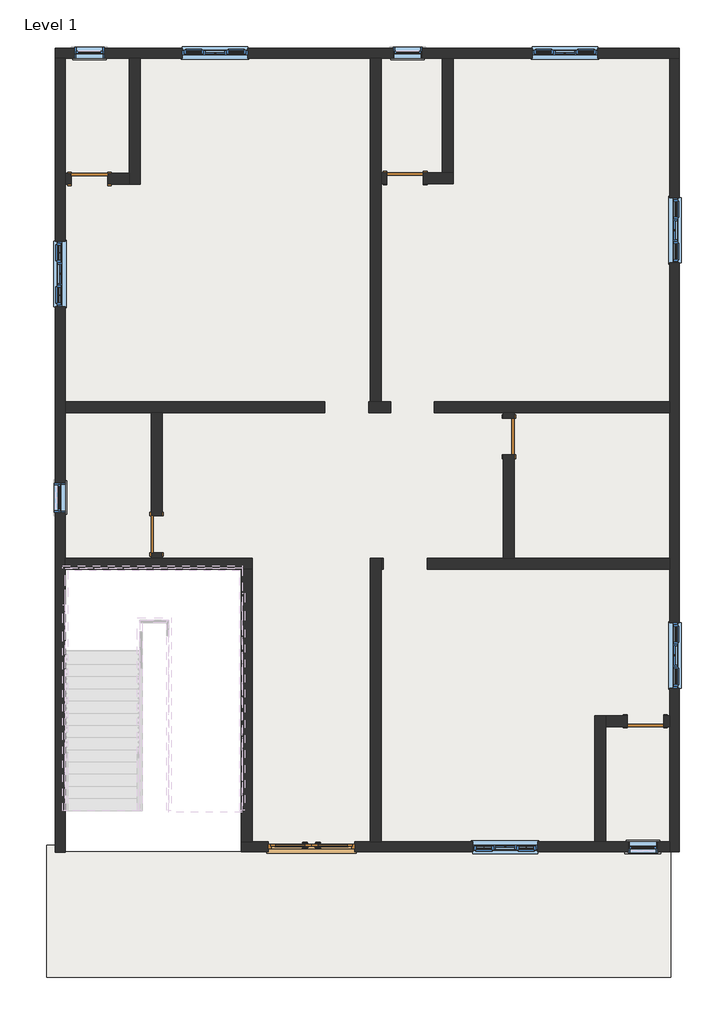
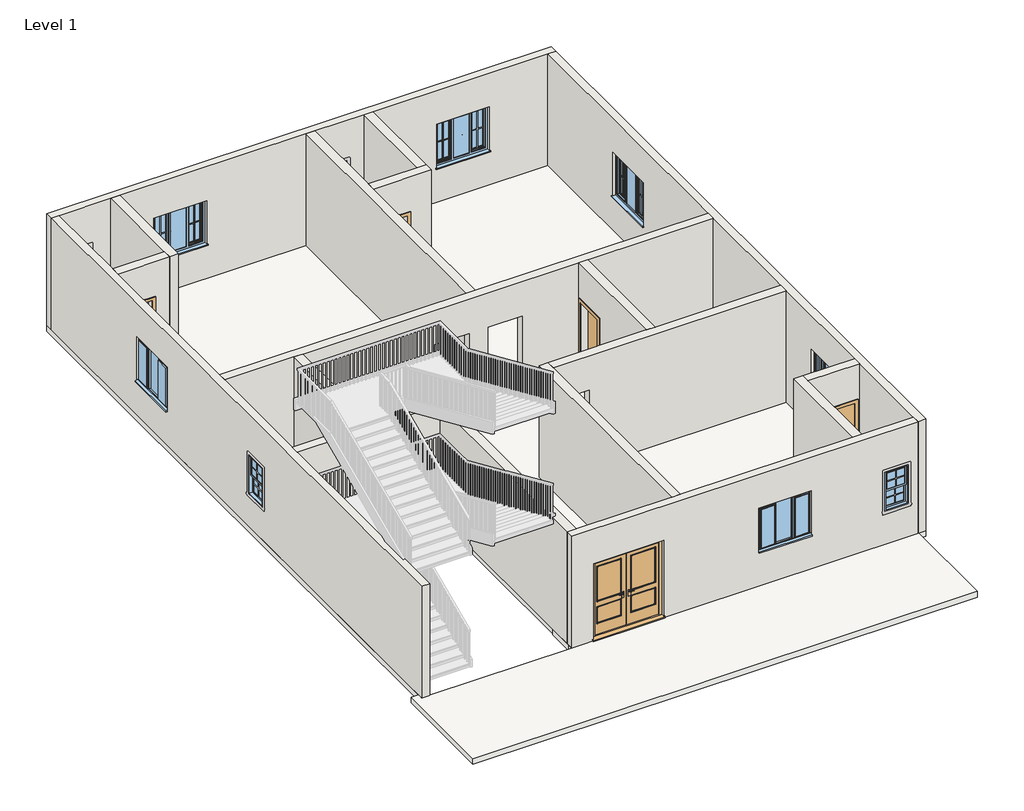
# One storey, part 1 of 6: 18 walls, 10 windows, 6 doors, 2 slabs.
"""IFC4 building model written with IfcOpenShell, lengths in millimetres."""

from ifc_helpers import new_model, si_unit, frame, origin, origin_with_axes, place, context, project, spatial, polyline, outline, extrude, faceted_brep, transform, mapped, element, save
from components import doors_extdbl_2_1810x2110mm_9ab1935a, doors_extdbl_2_1810x2110mm_b7024f51, door_85036156, window_679d2811, windows_tpl_w_glazing_cross_bars_1360x1210mm_0306471f

model = new_model("IFC4")

# Units and contexts
model_context = context("Model", 3, world=origin())
ifc_project = project(units=[si_unit("LENGTHUNIT", "METRE", prefix="MILLI")], contexts=[model_context])

# Site, building, storey
site = spatial("IfcSite", under=ifc_project)
building = spatial("IfcBuilding", under=site)
storey = spatial("IfcBuildingStorey", under=building, Name="Level 1", Elevation=0.0)

# Doors
placement = place(None, origin())
doors_extdbl_2_1810x2110mm_shape = doors_extdbl_2_1810x2110mm_9ab1935a(model_context)
doors_extdbl_2_1810x2110mm_2_shape = doors_extdbl_2_1810x2110mm_b7024f51(model_context)
element("IfcDoor", 1, ObjectType="Doors_ExtDbl_2 : 1810x2110mm", at=placement, inside=storey, context=model_context, shape_type="MappedRepresentation", body=[
    mapped(doors_extdbl_2_1810x2110mm_shape, transform((-2421.0852725, -7729.5064015, 0.0), x_axis=(1.0, 0.0, 0.0), y_axis=(0.0, 1.0, 0.0), z_axis=(0.0, 0.0, 1.0))),
    mapped(doors_extdbl_2_1810x2110mm_2_shape, transform((-2421.0852725, -7729.5064015, 0.0), x_axis=(1.0, 0.0, 0.0), y_axis=(0.0, 1.0, 0.0), z_axis=(0.0, 0.0, 1.0))),
])
door_shape = door_85036156(model_context)
element("IfcDoor", 2, ObjectType="Single-Flush : 30\" x 80\"", at=placement, inside=storey, context=model_context, shape_type="MappedRepresentation", body=[
    mapped(door_shape, transform((-7046.4415084, 6189.6935985, 0.0), x_axis=(-1.0, 0.0, 0.0), y_axis=(0.0, -1.0, 0.0), z_axis=(0.0, 0.0, 1.0))),
])
element("IfcDoor", 3, ObjectType="Single-Flush : 30\" x 80\"", at=placement, inside=storey, context=model_context, shape_type="MappedRepresentation", body=[
    mapped(door_shape, transform((-467.8415084, 6203.2000968, 0.0), x_axis=(-1.0, 0.0, 0.0), y_axis=(0.0, -1.0, 0.0), z_axis=(0.0, 0.0, 1.0))),
])
element("IfcDoor", 4, ObjectType="Single-Flush : 30\" x 80\"", at=placement, inside=storey, context=model_context, shape_type="MappedRepresentation", body=[
    mapped(door_shape, transform((-5649.4415084, -1217.2217109, 0.0), x_axis=(0.0, -1.0, 0.0), y_axis=(1.0, 0.0, 0.0), z_axis=(0.0, 0.0, 1.0))),
])
element("IfcDoor", 5, ObjectType="Single-Flush : 30\" x 80\"", at=placement, inside=storey, context=model_context, shape_type="MappedRepresentation", body=[
    mapped(door_shape, transform((1691.1584916, 817.5935985, 0.0), x_axis=(0.0, 1.0, 0.0), y_axis=(-1.0, 0.0, 0.0), z_axis=(0.0, 0.0, 1.0))),
])
element("IfcDoor", 6, ObjectType="Single-Flush : 30\" x 80\"", at=placement, inside=storey, context=model_context, shape_type="MappedRepresentation", body=[
    mapped(door_shape, transform((4535.9584916, -5113.3064015, 0.0), x_axis=(1.0, 0.0, 0.0), y_axis=(0.0, 1.0, 0.0), z_axis=(0.0, 0.0, 1.0))),
])

# Slabs
element("IfcSlab", 7, ObjectType="Generic - 12\"", at=placement, inside=storey, context=model_context, shape_type="SweptSolid", body=[
    extrude(outline(polyline([(5247.1584916, 8907.4935985), (5247.1584916, -7831.1064015), (-3879.0290366, -7831.1064015), (-3879.0290366, -6973.0610642), (-3866.3290366, -6973.0610642), (-3866.3290366, -1928.4217109), (-7554.4415084, -1928.4217109), (-7554.4415084, -7831.1064015), (-7757.6415084, -7831.1064015), (-7757.6415084, 8907.4935985), (5247.1584916, 8907.4935985)])), frame((0.0, 0.0, -152.4), z_axis=(0.0, 0.0, 1.0), x_axis=(1.0, 0.0, 0.0)), (0.0, 0.0, 1.0), 152.4),
])
element("IfcSlab", 8, ObjectType="Generic - 12\"", at=placement, inside=storey, context=model_context, shape_type="SweptSolid", body=[
    extrude(outline(polyline([(5063.8122085, -7701.6194881), (5063.8122085, -10451.1270757), (-7940.9877915, -10451.1270757), (-7940.9877915, -7701.6194881), (-7554.4415084, -7701.6194881), (-7554.4415084, -7831.1064015), (-3879.0290366, -7831.1064015), (-3879.0290366, -7701.6194881), (5063.8122085, -7701.6194881)])), frame((0.0, 0.0, -152.4), z_axis=(0.0, 0.0, 1.0), x_axis=(1.0, 0.0, 0.0)), (0.0, 0.0, 1.0), 152.4),
])

# Walls
element("IfcWall", 9, ObjectType="Generic - 4.5\"", at=placement, inside=storey, context=model_context, shape_type="Brep", body=[
    faceted_brep([(-1232.0415084, 1312.8935985, 2110.0), (-1232.0415084, 1312.8935985, 0.0), (-770.4415084, 1312.8935985, 0.0), (-770.4415084, 1312.8935985, 2110.0), (139.5584916, 1312.8935985, 2110.0), (139.5584916, 1312.8935985, 0.0), (1576.8584916, 1312.8935985, 0.0), (1805.4584916, 1312.8935985, 0.0), (5043.9584916, 1312.8935985, 0.0), (5043.9584916, 1312.8935985, 3048.0), (1805.4584916, 1312.8935985, 3048.0), (1576.8584916, 1312.8935985, 3048.0), (-5535.1415084, 1312.8935985, 3048.0), (-5763.7415084, 1312.8935985, 3048.0), (-7554.4415084, 1312.8935985, 3048.0), (-7554.4415084, 1312.8935985, 0.0), (-5763.7415084, 1312.8935985, 0.0), (-5535.1415084, 1312.8935985, 0.0), (-2142.0415084, 1312.8935985, 0.0), (-2142.0415084, 1312.8935985, 2110.0), (-770.4415084, 1541.4935985, 0.0), (-963.1415084, 1541.4935985, 0.0), (-1191.7415084, 1541.4935985, 0.0), (-1232.0415084, 1541.4935985, 0.0), (-1232.0415084, 1541.4935985, 2110.0), (-2142.0415084, 1541.4935985, 2110.0), (-2142.0415084, 1541.4935985, 0.0), (-7554.4415084, 1541.4935985, 0.0), (-7554.4415084, 1541.4935985, 3048.0), (-1191.7415084, 1541.4935985, 3048.0), (-963.1415084, 1541.4935985, 3048.0), (5043.9584916, 1541.4935985, 3048.0), (5043.9584916, 1541.4935985, 0.0), (139.5584916, 1541.4935985, 0.0), (139.5584916, 1541.4935985, 2110.0), (-770.4415084, 1541.4935985, 2110.0)], [[[0, 1, 2, 3, 4, 5, 6, 7, 8, 9, 10, 11, 12, 13, 14, 15, 16, 17, 18, 19]], [[20, 21, 22, 23, 24, 25, 26, 27, 28, 29, 30, 31, 32, 33, 34, 35]], [[33, 32, 8, 7, 6, 5]], [[2, 1, 23, 22, 21, 20]], [[18, 17, 16, 15, 27, 26]], [[14, 13, 12, 11, 10, 9, 31, 30, 29, 28]], [[9, 8, 32, 31]], [[15, 14, 28, 27]], [[5, 4, 34, 33]], [[3, 2, 20, 35]], [[4, 3, 35, 34]], [[26, 25, 19, 18]], [[24, 23, 1, 0]], [[25, 24, 0, 19]]]),
])
element("IfcWall", 10, ObjectType="Generic - 4.5\"", at=placement, inside=storey, context=model_context, shape_type="Brep", body=[
    faceted_brep([(-1191.7415084, 8704.2935985, 0.0), (-1191.7415084, 1541.4935985, 0.0), (-1191.7415084, 1541.4935985, 3048.0), (-1191.7415084, 8704.2935985, 3048.0), (-963.1415084, 8704.2935985, 0.0), (-963.1415084, 8704.2935985, 3048.0), (-963.1415084, 6317.5000968, 3048.0), (-963.1415084, 6088.9000968, 3048.0), (-963.1415084, 1541.4935985, 3048.0), (-963.1415084, 1541.4935985, 0.0), (-963.1415084, 6088.9000968, 0.0), (-963.1415084, 6317.5000968, 0.0)], [[[0, 1, 2, 3]], [[4, 5, 6, 7, 8, 9, 10, 11]], [[1, 0, 4, 11, 10, 9]], [[3, 2, 8, 7, 6, 5]], [[0, 3, 5, 4]], [[2, 1, 9, 8]]]),
])
element("IfcWall", 11, ObjectType="Generic - 4.5\"", at=placement, inside=storey, context=model_context, shape_type="Brep", body=[
    faceted_brep([(-6220.9415084, 8704.2935985, 0.0), (-6220.9415084, 6303.9935985, 0.0), (-6220.9415084, 6075.3935985, 0.0), (-6220.9415084, 6075.3935985, 3048.0), (-6220.9415084, 6303.9935985, 3048.0), (-6220.9415084, 8704.2935985, 3048.0), (-5992.3415084, 8704.2935985, 0.0), (-5992.3415084, 8704.2935985, 3048.0), (-5992.3415084, 6075.3935985, 3048.0), (-5992.3415084, 6075.3935985, 0.0)], [[[0, 1, 2, 3, 4, 5]], [[6, 7, 8, 9]], [[2, 1, 0, 6, 9]], [[5, 4, 3, 8, 7]], [[0, 5, 7, 6]], [[3, 2, 9, 8]]]),
])
element("IfcWall", 12, ObjectType="Generic - 4.5\"", at=placement, inside=storey, context=model_context, shape_type="SweptSolid", body=[
    extrude(outline(polyline([(0.0, -7554.4415084), (0.0, -7427.4415084), (2032.0, -7427.4415084), (2032.0, -6665.4415084), (0.0, -6665.4415084), (0.0, -6220.9415084), (3048.0, -6220.9415084), (3048.0, -7554.4415084), (0.0, -7554.4415084)])), frame((0.0, 6075.3935985, 0.0), z_axis=(0.0, 1.0, 0.0), x_axis=(0.0, 0.0, 1.0)), (0.0, 0.0, 1.0), 228.6),
])
element("IfcWall", 13, ObjectType="Generic - 4.5\"", at=placement, inside=storey, context=model_context, shape_type="Brep", body=[
    faceted_brep([(-963.1415084, 6088.9000968, 0.0), (-848.8415084, 6088.9000968, 0.0), (-848.8415084, 6088.9000968, 2032.0), (-86.8415084, 6088.9000968, 2032.0), (-86.8415084, 6088.9000968, 0.0), (535.4584916, 6088.9000968, 0.0), (535.4584916, 6088.9000968, 3048.0), (-963.1415084, 6088.9000968, 3048.0), (-848.8415084, 6317.5000968, 2032.0), (-848.8415084, 6317.5000968, 0.0), (-963.1415084, 6317.5000968, 0.0), (-963.1415084, 6317.5000968, 3048.0), (306.8584916, 6317.5000968, 3048.0), (535.4584916, 6317.5000968, 3048.0), (535.4584916, 6317.5000968, 0.0), (306.8584916, 6317.5000968, 0.0), (-86.8415084, 6317.5000968, 0.0), (-86.8415084, 6317.5000968, 2032.0)], [[[0, 1, 2, 3, 4, 5, 6, 7]], [[8, 9, 10, 11, 12, 13, 14, 15, 16, 17]], [[10, 9, 1, 0]], [[16, 15, 14, 5, 4]], [[7, 6, 13, 12, 11]], [[0, 7, 11, 10]], [[6, 5, 14, 13]], [[2, 1, 9, 8]], [[3, 2, 8, 17]], [[4, 3, 17, 16]]]),
])
element("IfcWall", 14, ObjectType="Generic - 4.5\"", at=placement, inside=storey, context=model_context, shape_type="SweptSolid", body=[
    extrude(outline(polyline([(535.4584916, 8704.2935985), (535.4584916, 6317.5000968), (306.8584916, 6317.5000968), (306.8584916, 8704.2935985), (535.4584916, 8704.2935985)])), origin_with_axes(), (0.0, 0.0, 1.0), 3048.0),
])
element("IfcWall", 15, ObjectType="Generic - 4.5\"", at=placement, inside=storey, context=model_context, shape_type="SweptSolid", body=[
    extrude(outline(polyline([(-1598.2217109, 2032.0), (-1598.2217109, 0.0), (-1712.5217109, 0.0), (-1712.5217109, 3048.0), (1312.8935985, 3048.0), (1312.8935985, 0.0), (-836.2217109, 0.0), (-836.2217109, 2032.0), (-1598.2217109, 2032.0)])), frame((-5763.7415084, 0.0, 0.0), z_axis=(1.0, 0.0, 0.0), x_axis=(0.0, 1.0, 0.0)), (0.0, 0.0, 1.0), 228.6),
])
element("IfcWall", 16, ObjectType="Generic - 4.5\"", at=placement, inside=storey, context=model_context, shape_type="Brep", body=[
    faceted_brep([(-7554.4415084, -1941.1217109, 0.0), (-3879.0290366, -1941.1217109, 0.0), (-3650.4290366, -1941.1217109, 0.0), (-3650.4290366, -1941.1217109, 3048.0), (-3879.0290366, -1941.1217109, 3048.0), (-7554.4415084, -1941.1217109, 3048.0), (-7554.4415084, -1712.5217109, 0.0), (-7554.4415084, -1712.5217109, 3048.0), (-5763.7415084, -1712.5217109, 3048.0), (-5535.1415084, -1712.5217109, 3048.0), (-3650.4290366, -1712.5217109, 3048.0), (-3650.4290366, -1712.5217109, 0.0), (-5535.1415084, -1712.5217109, 0.0), (-5763.7415084, -1712.5217109, 0.0)], [[[0, 1, 2, 3, 4, 5]], [[6, 7, 8, 9, 10, 11, 12, 13]], [[2, 1, 0, 6, 13, 12, 11]], [[5, 4, 3, 10, 9, 8, 7]], [[0, 5, 7, 6]], [[3, 2, 11, 10]]]),
])
element("IfcWall", 17, ObjectType="Generic - 4.5\"", at=placement, inside=storey, context=model_context, shape_type="SweptSolid", body=[
    extrude(outline(polyline([(-3879.0290366, -7627.9064015), (-3879.0290366, -1941.1217109), (-3650.4290366, -1941.1217109), (-3650.4290366, -7627.9064015), (-3879.0290366, -7627.9064015)])), origin_with_axes(), (0.0, 0.0, 1.0), 3048.0),
])
element("IfcWall", 18, ObjectType="Generic - 4.5\"", at=placement, inside=storey, context=model_context, shape_type="SweptSolid", body=[
    extrude(outline(polyline([(1312.8935985, 0.0), (1198.5935985, 0.0), (1198.5935985, 2032.0), (436.5935985, 2032.0), (436.5935985, 0.0), (-1712.5217109, 0.0), (-1712.5217109, 3048.0), (1312.8935985, 3048.0), (1312.8935985, 0.0)])), frame((1576.8584916, 0.0, 0.0), z_axis=(1.0, 0.0, 0.0), x_axis=(0.0, 1.0, 0.0)), (0.0, 0.0, 1.0), 228.6),
])
element("IfcWall", 19, ObjectType="Generic - 4.5\"", at=placement, inside=storey, context=model_context, shape_type="Brep", body=[
    faceted_brep([(-963.1415084, -7627.9064015, 0.0), (-963.1415084, -1941.1217109, 0.0), (-963.1415084, -1712.5217109, 0.0), (-963.1415084, -1712.5217109, 3048.0), (-963.1415084, -1941.1217109, 3048.0), (-963.1415084, -7627.9064015, 3048.0), (-1191.7415084, -7627.9064015, 0.0), (-1191.7415084, -7627.9064015, 3048.0), (-1191.7415084, -1712.5217109, 3048.0), (-1191.7415084, -1712.5217109, 0.0)], [[[0, 1, 2, 3, 4, 5]], [[6, 7, 8, 9]], [[2, 1, 0, 6, 9]], [[5, 4, 3, 8, 7]], [[0, 5, 7, 6]], [[3, 2, 9, 8]]]),
])
element("IfcWall", 20, ObjectType="Generic - 4.5\"", at=placement, inside=storey, context=model_context, shape_type="Brep", body=[
    faceted_brep([(-922.8415084, -1712.5217109, 2110.0), (-922.8415084, -1712.5217109, 0.0), (-963.1415084, -1712.5217109, 0.0), (-963.1415084, -1712.5217109, 3048.0), (1576.8584916, -1712.5217109, 3048.0), (1805.4584916, -1712.5217109, 3048.0), (5043.9584916, -1712.5217109, 3048.0), (5043.9584916, -1712.5217109, 0.0), (1805.4584916, -1712.5217109, 0.0), (1576.8584916, -1712.5217109, 0.0), (-12.8415084, -1712.5217109, 0.0), (-12.8415084, -1712.5217109, 2110.0), (-963.1415084, -1941.1217109, 0.0), (-922.8415084, -1941.1217109, 0.0), (-922.8415084, -1941.1217109, 2110.0), (-12.8415084, -1941.1217109, 2110.0), (-12.8415084, -1941.1217109, 0.0), (5043.9584916, -1941.1217109, 0.0), (5043.9584916, -1941.1217109, 3048.0), (-963.1415084, -1941.1217109, 3048.0)], [[[0, 1, 2, 3, 4, 5, 6, 7, 8, 9, 10, 11]], [[12, 13, 14, 15, 16, 17, 18, 19]], [[2, 1, 13, 12]], [[10, 9, 8, 7, 17, 16]], [[6, 5, 4, 3, 19, 18]], [[3, 2, 12, 19]], [[7, 6, 18, 17]], [[16, 15, 11, 10]], [[14, 13, 1, 0]], [[15, 14, 0, 11]]]),
])
element("IfcWall", 21, ObjectType="Generic - 4.5\"", at=placement, inside=storey, context=model_context, shape_type="Brep", body=[
    faceted_brep([(3710.4584916, -7627.9064015, 0.0), (3710.4584916, -5227.6064015, 0.0), (3710.4584916, -4999.0064015, 0.0), (3710.4584916, -4999.0064015, 3048.0), (3710.4584916, -5227.6064015, 3048.0), (3710.4584916, -7627.9064015, 3048.0), (3481.8584916, -7627.9064015, 0.0), (3481.8584916, -7627.9064015, 3048.0), (3481.8584916, -4999.0064015, 3048.0), (3481.8584916, -4999.0064015, 0.0)], [[[0, 1, 2, 3, 4, 5]], [[6, 7, 8, 9]], [[2, 1, 0, 6, 9]], [[5, 4, 3, 8, 7]], [[0, 5, 7, 6]], [[3, 2, 9, 8]]]),
])
element("IfcWall", 22, ObjectType="Generic - 4.5\"", at=placement, inside=storey, context=model_context, shape_type="SweptSolid", body=[
    extrude(outline(polyline([(2032.0, 4916.9584916), (0.0, 4916.9584916), (0.0, 5043.9584916), (3048.0, 5043.9584916), (3048.0, 3710.4584916), (0.0, 3710.4584916), (0.0, 4154.9584916), (2032.0, 4154.9584916), (2032.0, 4916.9584916)])), frame((0.0, -5227.6064015, 0.0), z_axis=(0.0, 1.0, 0.0), x_axis=(0.0, 0.0, 1.0)), (0.0, 0.0, 1.0), 228.6),
])
element("IfcWall", 23, ObjectType="Generic - 9\"", at=placement, inside=storey, context=model_context, shape_type="Brep", body=[
    faceted_brep([(-7757.6415084, 8704.2935985, 0.0), (-7554.4415084, 8704.2935985, 0.0), (-6220.9415084, 8704.2935985, 0.0), (-5992.3415084, 8704.2935985, 0.0), (-1191.7415084, 8704.2935985, 0.0), (-963.1415084, 8704.2935985, 0.0), (306.8584916, 8704.2935985, 0.0), (535.4584916, 8704.2935985, 0.0), (5043.9584916, 8704.2935985, 0.0), (5247.1584916, 8704.2935985, 0.0), (5247.1584916, 8704.2935985, 3048.0), (5043.9584916, 8704.2935985, 3048.0), (535.4584916, 8704.2935985, 3048.0), (306.8584916, 8704.2935985, 3048.0), (-963.1415084, 8704.2935985, 3048.0), (-1191.7415084, 8704.2935985, 3048.0), (-5992.3415084, 8704.2935985, 3048.0), (-6220.9415084, 8704.2935985, 3048.0), (-7554.4415084, 8704.2935985, 3048.0), (-7757.6415084, 8704.2935985, 3048.0), (2179.5584916, 8704.2935985, 2124.4), (3539.5584916, 8704.2935985, 2124.4), (3539.5584916, 8704.2935985, 914.4), (2179.5584916, 8704.2935985, 914.4), (-5110.2415084, 8704.2935985, 2124.4), (-3750.2415084, 8704.2935985, 2124.4), (-3750.2415084, 8704.2935985, 914.4), (-5110.2415084, 8704.2935985, 914.4), (-7351.2415084, 8704.2935985, 1981.2), (-6741.6415084, 8704.2935985, 1981.2), (-6741.6415084, 8704.2935985, 914.4), (-7351.2415084, 8704.2935985, 914.4), (-721.8415084, 8704.2935985, 1981.2), (-112.2415084, 8704.2935985, 1981.2), (-112.2415084, 8704.2935985, 914.4), (-721.8415084, 8704.2935985, 914.4), (-7757.6415084, 8907.4935985, 0.0), (-7757.6415084, 8907.4935985, 3048.0), (5247.1584916, 8907.4935985, 3048.0), (5247.1584916, 8907.4935985, 0.0), (2179.5584916, 8907.4935985, 2124.4), (2179.5584916, 8907.4935985, 914.4), (3539.5584916, 8907.4935985, 914.4), (3539.5584916, 8907.4935985, 2124.4), (-5110.2415084, 8907.4935985, 2124.4), (-5110.2415084, 8907.4935985, 914.4), (-3750.2415084, 8907.4935985, 914.4), (-3750.2415084, 8907.4935985, 2124.4), (-7351.2415084, 8907.4935985, 1981.2), (-7351.2415084, 8907.4935985, 914.4), (-6741.6415084, 8907.4935985, 914.4), (-6741.6415084, 8907.4935985, 1981.2), (-721.8415084, 8907.4935985, 1981.2), (-721.8415084, 8907.4935985, 914.4), (-112.2415084, 8907.4935985, 914.4), (-112.2415084, 8907.4935985, 1981.2)], [[[0, 1, 2, 3, 4, 5, 6, 7, 8, 9, 10, 11, 12, 13, 14, 15, 16, 17, 18, 19], [20, 21, 22, 23], [24, 25, 26, 27], [28, 29, 30, 31], [32, 33, 34, 35]], [[36, 37, 38, 39], [40, 41, 42, 43], [44, 45, 46, 47], [48, 49, 50, 51], [52, 53, 54, 55]], [[9, 8, 7, 6, 5, 4, 3, 2, 1, 0, 36, 39]], [[19, 18, 17, 16, 15, 14, 13, 12, 11, 10, 38, 37]], [[0, 19, 37, 36]], [[10, 9, 39, 38]], [[41, 40, 20, 23]], [[42, 41, 23, 22]], [[43, 42, 22, 21]], [[40, 43, 21, 20]], [[45, 44, 24, 27]], [[46, 45, 27, 26]], [[47, 46, 26, 25]], [[44, 47, 25, 24]], [[49, 48, 28, 31]], [[50, 49, 31, 30]], [[51, 50, 30, 29]], [[48, 51, 29, 28]], [[53, 52, 32, 35]], [[54, 53, 35, 34]], [[55, 54, 34, 33]], [[52, 55, 33, 32]]]),
])
element("IfcWall", 24, ObjectType="Generic - 9\"", at=placement, inside=storey, context=model_context, shape_type="Brep", body=[
    faceted_brep([(5043.9584916, 8704.2935985, 0.0), (5043.9584916, 1541.4935985, 0.0), (5043.9584916, 1312.8935985, 0.0), (5043.9584916, -1712.5217109, 0.0), (5043.9584916, -1941.1217109, 0.0), (5043.9584916, -4999.0064015, 0.0), (5043.9584916, -5227.6064015, 0.0), (5043.9584916, -7627.9064015, 0.0), (5043.9584916, -7831.1064015, 0.0), (5043.9584916, -7831.1064015, 3048.0), (5043.9584916, -7627.9064015, 3048.0), (5043.9584916, -5227.6064015, 3048.0), (5043.9584916, -4999.0064015, 3048.0), (5043.9584916, -1941.1217109, 3048.0), (5043.9584916, -1712.5217109, 3048.0), (5043.9584916, 1312.8935985, 3048.0), (5043.9584916, 1541.4935985, 3048.0), (5043.9584916, 8704.2935985, 3048.0), (5043.9584916, 5796.5435985, 2124.4), (5043.9584916, 4436.5435985, 2124.4), (5043.9584916, 4436.5435985, 914.4), (5043.9584916, 5796.5435985, 914.4), (5043.9584916, -3061.7064015, 2124.4), (5043.9584916, -4421.7064015, 2124.4), (5043.9584916, -4421.7064015, 914.4), (5043.9584916, -3061.7064015, 914.4), (5247.1584916, 8704.2935985, 0.0), (5247.1584916, 8704.2935985, 3048.0), (5247.1584916, -7831.1064015, 3048.0), (5247.1584916, -7831.1064015, 0.0), (5247.1584916, 5796.5435985, 2124.4), (5247.1584916, 5796.5435985, 914.4), (5247.1584916, 4436.5435985, 914.4), (5247.1584916, 4436.5435985, 2124.4), (5247.1584916, -3061.7064015, 2124.4), (5247.1584916, -3061.7064015, 914.4), (5247.1584916, -4421.7064015, 914.4), (5247.1584916, -4421.7064015, 2124.4)], [[[0, 1, 2, 3, 4, 5, 6, 7, 8, 9, 10, 11, 12, 13, 14, 15, 16, 17], [18, 19, 20, 21], [22, 23, 24, 25]], [[26, 27, 28, 29], [30, 31, 32, 33], [34, 35, 36, 37]], [[8, 7, 6, 5, 4, 3, 2, 1, 0, 26, 29]], [[9, 8, 29, 28]], [[17, 16, 15, 14, 13, 12, 11, 10, 9, 28, 27]], [[31, 30, 18, 21]], [[32, 31, 21, 20]], [[33, 32, 20, 19]], [[30, 33, 19, 18]], [[35, 34, 22, 25]], [[36, 35, 25, 24]], [[37, 36, 24, 23]], [[34, 37, 23, 22]], [[0, 17, 27, 26]]]),
])
element("IfcWall", 25, ObjectType="Generic - 9\"", at=placement, inside=storey, context=model_context, shape_type="Brep", body=[
    faceted_brep([(5043.9584916, -7627.9064015, 0.0), (3710.4584916, -7627.9064015, 0.0), (3481.8584916, -7627.9064015, 0.0), (-963.1415084, -7627.9064015, 0.0), (-1191.7415084, -7627.9064015, 0.0), (-1516.0852725, -7627.9064015, 0.0), (-1516.0852725, -7627.9064015, 2110.0), (-3326.0852725, -7627.9064015, 2110.0), (-3326.0852725, -7627.9064015, 0.0), (-3650.4290366, -7627.9064015, 0.0), (-3879.0290366, -7627.9064015, 0.0), (-3879.0290366, -7627.9064015, 3048.0), (-3650.4290366, -7627.9064015, 3048.0), (-1191.7415084, -7627.9064015, 3048.0), (-963.1415084, -7627.9064015, 3048.0), (3481.8584916, -7627.9064015, 3048.0), (3710.4584916, -7627.9064015, 3048.0), (5043.9584916, -7627.9064015, 3048.0), (2294.9584916, -7627.9064015, 2124.4), (934.9584916, -7627.9064015, 2124.4), (934.9584916, -7627.9064015, 914.4), (2294.9584916, -7627.9064015, 914.4), (4789.9584916, -7627.9064015, 1981.2), (4180.3584916, -7627.9064015, 1981.2), (4180.3584916, -7627.9064015, 914.4), (4789.9584916, -7627.9064015, 914.4), (-1516.0852725, -7831.1064015, 2110.0), (-1516.0852725, -7831.1064015, 0.0), (5043.9584916, -7831.1064015, 0.0), (5043.9584916, -7831.1064015, 3048.0), (-3879.0290366, -7831.1064015, 3048.0), (-3879.0290366, -7831.1064015, 0.0), (-3326.0852725, -7831.1064015, 0.0), (-3326.0852725, -7831.1064015, 2110.0), (2294.9584916, -7831.1064015, 2124.4), (2294.9584916, -7831.1064015, 914.4), (934.9584916, -7831.1064015, 914.4), (934.9584916, -7831.1064015, 2124.4), (4789.9584916, -7831.1064015, 1981.2), (4789.9584916, -7831.1064015, 914.4), (4180.3584916, -7831.1064015, 914.4), (4180.3584916, -7831.1064015, 1981.2)], [[[0, 1, 2, 3, 4, 5, 6, 7, 8, 9, 10, 11, 12, 13, 14, 15, 16, 17], [18, 19, 20, 21], [22, 23, 24, 25]], [[26, 27, 28, 29, 30, 31, 32, 33], [34, 35, 36, 37], [38, 39, 40, 41]], [[32, 31, 10, 9, 8]], [[28, 27, 5, 4, 3, 2, 1, 0]], [[17, 16, 15, 14, 13, 12, 11, 30, 29]], [[0, 17, 29, 28]], [[11, 10, 31, 30]], [[35, 34, 18, 21]], [[36, 35, 21, 20]], [[37, 36, 20, 19]], [[34, 37, 19, 18]], [[39, 38, 22, 25]], [[40, 39, 25, 24]], [[41, 40, 24, 23]], [[38, 41, 23, 22]], [[8, 7, 33, 32]], [[6, 5, 27, 26]], [[7, 6, 26, 33]]]),
])
element("IfcWall", 26, ObjectType="Generic - 9\"", at=placement, inside=storey, context=model_context, shape_type="Brep", body=[
    faceted_brep([(-7757.6415084, 8704.2935985, 0.0), (-7757.6415084, -7843.8064015, 0.0), (-7757.6415084, -7843.8064015, 3048.0), (-7757.6415084, 8704.2935985, 3048.0), (-7757.6415084, 3528.4935985, 2124.4), (-7757.6415084, 3528.4935985, 914.4), (-7757.6415084, 4888.4935985, 914.4), (-7757.6415084, 4888.4935985, 2124.4), (-7757.6415084, -760.0217109, 1981.2), (-7757.6415084, -760.0217109, 914.4), (-7757.6415084, -150.4217109, 914.4), (-7757.6415084, -150.4217109, 1981.2), (-7554.4415084, 8704.2935985, 0.0), (-7554.4415084, 8704.2935985, 3048.0), (-7554.4415084, 6303.9935985, 3048.0), (-7554.4415084, 6075.3935985, 3048.0), (-7554.4415084, 1541.4935985, 3048.0), (-7554.4415084, 1312.8935985, 3048.0), (-7554.4415084, -1712.5217109, 3048.0), (-7554.4415084, -1941.1217109, 3048.0), (-7554.4415084, -7843.8064015, 3048.0), (-7554.4415084, -7843.8064015, 0.0), (-7554.4415084, -1941.1217109, 0.0), (-7554.4415084, -1712.5217109, 0.0), (-7554.4415084, 1312.8935985, 0.0), (-7554.4415084, 1541.4935985, 0.0), (-7554.4415084, 6075.3935985, 0.0), (-7554.4415084, 6303.9935985, 0.0), (-7554.4415084, 3528.4935985, 2124.4), (-7554.4415084, 4888.4935985, 2124.4), (-7554.4415084, 4888.4935985, 914.4), (-7554.4415084, 3528.4935985, 914.4), (-7554.4415084, -760.0217109, 1981.2), (-7554.4415084, -150.4217109, 1981.2), (-7554.4415084, -150.4217109, 914.4), (-7554.4415084, -760.0217109, 914.4)], [[[0, 1, 2, 3], [4, 5, 6, 7], [8, 9, 10, 11]], [[12, 13, 14, 15, 16, 17, 18, 19, 20, 21, 22, 23, 24, 25, 26, 27], [28, 29, 30, 31], [32, 33, 34, 35]], [[1, 0, 12, 27, 26, 25, 24, 23, 22, 21]], [[2, 1, 21, 20]], [[3, 2, 20, 19, 18, 17, 16, 15, 14, 13]], [[0, 3, 13, 12]], [[5, 4, 28, 31]], [[6, 5, 31, 30]], [[7, 6, 30, 29]], [[4, 7, 29, 28]], [[9, 8, 32, 35]], [[10, 9, 35, 34]], [[11, 10, 34, 33]], [[8, 11, 33, 32]]]),
])

# Windows
window_shape = window_679d2811(model_context)
element("IfcWindow", 27, ObjectType="Window-Double-Hung : 24\" x 42\"", at=placement, inside=storey, context=model_context, shape_type="MappedRepresentation", body=[
    mapped(window_shape, transform((-7656.0415084, -455.2217109, 0.0), x_axis=(0.0, 1.0, 0.0), y_axis=(-1.0, 0.0, 0.0), z_axis=(0.0, 0.0, 1.0))),
])
element("IfcWindow", 28, ObjectType="Window-Double-Hung : 24\" x 42\"", at=placement, inside=storey, context=model_context, shape_type="MappedRepresentation", body=[
    mapped(window_shape, transform((-7046.4415084, 8805.8935985, 0.0), x_axis=(1.0, 0.0, 0.0), y_axis=(0.0, 1.0, 0.0), z_axis=(0.0, 0.0, 1.0))),
])
element("IfcWindow", 29, ObjectType="Window-Double-Hung : 24\" x 42\"", at=placement, inside=storey, context=model_context, shape_type="MappedRepresentation", body=[
    mapped(window_shape, transform((-417.0415084, 8805.8935985, 0.0), x_axis=(1.0, 0.0, 0.0), y_axis=(0.0, 1.0, 0.0), z_axis=(0.0, 0.0, 1.0))),
])
element("IfcWindow", 30, ObjectType="Window-Double-Hung : 24\" x 42\"", at=placement, inside=storey, context=model_context, shape_type="MappedRepresentation", body=[
    mapped(window_shape, transform((4485.1584916, -7729.5064015, 0.0), x_axis=(-1.0, 0.0, 0.0), y_axis=(0.0, -1.0, 0.0), z_axis=(0.0, 0.0, 1.0))),
])
windows_tpl_w_glazing_cross_bars_1360x1210mm_shape = windows_tpl_w_glazing_cross_bars_1360x1210mm_0306471f(model_context)
element("IfcWindow", 31, ObjectType="Windows_Tpl_w-Glazing_Cross-Bars : 1360x1210mm", at=placement, inside=storey, context=model_context, shape_type="MappedRepresentation", body=[
    mapped(windows_tpl_w_glazing_cross_bars_1360x1210mm_shape, transform((5137.1019238, 4614.8769318, 14.4), x_axis=(0.0, -1.0, 0.0), y_axis=(1.0, 0.0, 0.0), z_axis=(0.0, 0.0, 1.0))),
])
element("IfcWindow", 32, ObjectType="Windows_Tpl_w-Glazing_Cross-Bars : 1360x1210mm", at=placement, inside=storey, context=model_context, shape_type="MappedRepresentation", body=[
    mapped(windows_tpl_w_glazing_cross_bars_1360x1210mm_shape, transform((5137.1019238, -4243.3730682, 14.4), x_axis=(0.0, -1.0, 0.0), y_axis=(1.0, 0.0, 0.0), z_axis=(0.0, 0.0, 1.0))),
])
element("IfcWindow", 33, ObjectType="Windows_Tpl_w-Glazing_Cross-Bars : 1360x1210mm", at=placement, inside=storey, context=model_context, shape_type="MappedRepresentation", body=[
    mapped(windows_tpl_w_glazing_cross_bars_1360x1210mm_shape, transform((1113.2918249, -7721.0498337, 14.4), x_axis=(-1.0, 0.0, 0.0), y_axis=(0.0, -1.0, 0.0), z_axis=(0.0, 0.0, 1.0))),
])
element("IfcWindow", 34, ObjectType="Windows_Tpl_w-Glazing_Cross-Bars : 1360x1210mm", at=placement, inside=storey, context=model_context, shape_type="MappedRepresentation", body=[
    mapped(windows_tpl_w_glazing_cross_bars_1360x1210mm_shape, transform((3361.2251583, 8797.4370307, 14.4), x_axis=(1.0, 0.0, 0.0), y_axis=(0.0, 1.0, 0.0), z_axis=(0.0, 0.0, 1.0))),
])
element("IfcWindow", 35, ObjectType="Windows_Tpl_w-Glazing_Cross-Bars : 1360x1210mm", at=placement, inside=storey, context=model_context, shape_type="MappedRepresentation", body=[
    mapped(windows_tpl_w_glazing_cross_bars_1360x1210mm_shape, transform((-3928.5748417, 8797.4370307, 14.4), x_axis=(1.0, 0.0, 0.0), y_axis=(0.0, 1.0, 0.0), z_axis=(0.0, 0.0, 1.0))),
])
element("IfcWindow", 36, ObjectType="Windows_Tpl_w-Glazing_Cross-Bars : 1360x1210mm", at=placement, inside=storey, context=model_context, shape_type="MappedRepresentation", body=[
    mapped(windows_tpl_w_glazing_cross_bars_1360x1210mm_shape, transform((-7647.5849406, 4710.1602652, 14.4), x_axis=(0.0, 1.0, 0.0), y_axis=(-1.0, 0.0, 0.0), z_axis=(0.0, 0.0, 1.0))),
])

save(model, "model.ifc")

# Revit data of these elements
# Type "Doors_ExtDbl_2 : 1810x2110mm"
#   Type Mark = "8"
#   Type Comments = "External Double"
#   Operation = "DoubleDoorSingleSwing"
#   Construction Type Id = "GSP4R"
#   Keynote = "L20"
#   Analytic Construction = "1/8 in Pilkington single glazing"
#   Wrap Layers (Int) from Ext = 0' - 6.98819"
#   Wrap Layers (Ext) from Ext = 0' - 4.03543"
#   Visual Light Transmittance = 0.9
#   Top of Lock Rail = 2' - 11.43307"
#   Thickness = 0' - 1.73228"
#   Stile Shutting = 0' - 4.92126"
#   Stile - Top Rail = 0' - 5.90551"
#   Stile - Lock Rail = 0' - 5.90551"
#   Stile - Hanging = 0' - 3.93701"
#   Stile - Bottom Rail = 0' - 11.81102"
#   Solar Heat Gain Coefficient = 0.78
#   Rough Width = 5' - 11.25984"
#   Rough Height = 6' - 11.07087"
#   O/A Frame Width = 0' - 2.51969"
#   Heat Transfer Coefficient (U) = 0.6496 BTU/(h·ft²·°F)
#   Handle Z Distance = 3' - 1.40157"
#   Glazing Thickness = 0' - 0.94488"
#   FrameWidth = 0' - 1.65354"
#   FrameOffset - External = 0' - 2.55906"
#   FrameDepth = 0' - 3.50394"
#   Door Panel Width = 2' - 9.54331"
#   Door Panel Thickness = 0' - 1.73228"
#   Door Panel Height = 6' - 6.74016"
#   Cill Thickness = 0' - 2.14567"
#   Cill Projection = 0' - 1.1811"
#   Handle X Distance = 0' - 2.95276"
#   Height = 6' - 11.07087"
#   Structural Tolerance = 0' - 0.25591"
#   Tolerance = 0' - 0.11811"
#   Undercut = 0' - 0.15748"
#   Width = 5' - 11.25984"
#   Cill Extension = 0' - 0.98425"
#   Cavity Closer Width = 0' - 1.9685"
#   Cavity Closer Offset from Ext = 0' - 4.03543"
#   Cavity Closer Depth = 0' - 3.34646"
#   Vis - Ironmongery = yes
#   Vis - Cavity Closers = yes
#   Define Thermal Properties by = 1
#   Function = 1
#   Material Glass = Door - Glazing
#   Handle Style = element 387460
#   Material Door = Door - Panel
#   Material Frame = Door - Frame/Mullion
#   Material Ironmongery = Door - Handle
#   Wall Closure = (empty or 0)
# Type "Single-Flush : 30\" x 80\""
#   Type Mark = "5"
#   Construction Type Id = "MDOOR"
#   Assembly Code = "C1020"
#   Analytic Construction = "Metal"
#   Thickness = 0' - 2"
#   Heat Transfer Coefficient (U) = 0.651978 BTU/(h·ft²·°F)
#   Height = 6' - 8"
#   Trim Projection Ext = 0' - 1"
#   Trim Projection Int = 0' - 1"
#   Trim Width = 0' - 3"
#   Width = 2' - 6"
#   Define Thermal Properties by = 1
#   Define Thermal Properties by = 1
#   Door Material = Door - Panel
#   Frame Material = Door - Frame
#   Visual Light Transmittance = 0
#   Solar Heat Gain Coefficient = 0
#   Function = (empty or 0)
#   Wall Closure = (empty or 0)
# Type "Generic - 12\""
#   Assembly Code = "B1010"
#   Function = 0
#   Layers, outside or top first: 0' - 6" no material (function 1)
# Type "Generic - 4.5\""
#   Assembly Code = "B2010"
#   Layers, outside or top first: 0' - 9" no material (function 1)
# Type "Generic - 9\""
#   Assembly Code = "B2010"
#   Layers, outside or top first: 0' - 8" no material (function 1)
# Type "Window-Double-Hung : 24\" x 42\""
#   Type Mark = "10"
#   Fire Rating = "0.5h"
#   Construction Type Id = "DG-DR"
#   Assembly Code = "B2020100"
#   Analytic Construction = "Double glazing - domestic"
#   Wall Thickness [instance default] = 0' - 6"
#   Window Inset [instance default] = 0' - 0"
#   Visual Light Transmittance = 0.81
#   Thermal Resistance (R) = 1.8146 (h·ft²·°F)/BTU
#   Solar Heat Gain Coefficient = 0.76
#   Muntin Width = 1' - 6"
#   Muntin Height = 1' - 5 1/8"
#   Interior Wall Closure [instance default] = 0' - 1 1/2"
#   Rough Width = 2' - 0 1/2"
#   Rough Height = 3' - 6 1/2"
#   Frame Extension [instance default] = 0' - 1 1/4"
#   Exterior Wall Closure [instance default] = 0' - 0 1/2"
#   Extension Jamb [instance default] = 0' - 1 1/2"
#   Heat Transfer Coefficient (U) = 0.5511 BTU/(h·ft²·°F)
#   Height = 3' - 6"
#   Width = 2' - 0"
#   Define Thermal Properties by = 1
#   Top Muntin Visibility = yes
#   Indicator Visibility [instance default] = yes
#   Extension Jamb Visibility [instance default] = yes
#   Interior Trim Visibility [instance default] = yes
#   Exterior Trim Visibility [instance default] = yes
#   Define Thermal Properties by = 1
#   Bottom Muntin Visibility = yes
#   Muntin Pattern = Muntin Pattern_2x2 : Muntin Pattern_2x2
#   Interior Trim Material = Wood - Stained
#   Interior Trim = Trim-Window-Interior-Flat : Picture Frame
#   Exterior Trim Material = Clad - White
#   Exterior Trim = Trim-Window-Exterior-Flat : with Sill
#   Glass Panel Material = Glass
#   Exterior Frame Material = Clad - White
#   Interior Frame Material = Wood - Stained
#   Wall Closure = (empty or 0)
# Type "Windows_Tpl_w-Glazing_Cross-Bars : 1360x1210mm"
#   Type Mark = "21"
#   Operation = "TriplePanelVertical"
#   Construction Type Id = "GSP4R"
#   Manufacturer = "Revit"
#   Keynote = "L10"
#   Analytic Construction = "1/8 in Pilkington single glazing"
#   Wrap Layers (Ext) from Ext = 0' - 4.03543"
#   Wrap Layers (Int) from Ext = 0' - 6.98819"
#   Window Board Projection = 0' - 0.98425"
#   Window Board Extension = 0' - 0.98425"
#   Visual Light Transmittance = 0.9
#   Solar Heat Gain Coefficient = 0.78
#   Rough Width = 4' - 5.54331"
#   Rough Height = 3' - 11.6378"
#   Height = 3' - 11.6378"
#   Width = 4' - 5.54331"
#   Heat Transfer Coefficient (U) = 0.6496 BTU/(h·ft²·°F)
#   Glazing Thickness = 0' - 0.94488"
#   Glazing Bar Thickness = 0' - 0.7874"
#   FrameOffset - External = 0' - 1.9685"
#   Frame Depth = 0' - 2.55906"
#   Default Head Height = 6' - 11.07087"
#   Cill Depth = 0' - 3.44488"
#   Cavity Closer Width = 0' - 1.9685"
#   Cavity Closer Offset from Ext = 0' - 4.03543"
#   Cavity Closer Depth = 0' - 3.34646"
#   Vis - Glazing Bars = yes
#   Vis - Cavity Closers = yes
#   Define Thermal Properties by = 1
#   Material Trim = Window Frame
#   Material Glazing Bars = Window Frame
#   Material Glass = Glass
#   Material Frame = Window Frame
#   Wall Closure = (empty or 0)
# Element 1 (IfcDoor, "Doors_ExtDbl_2 : 1810x2110mm")
#   Phase Created = New Construction
#   Materials on its faces: "Door - Panel", "Door - Handle", "Door - Frame/Mullion", "Door - Glazing"
# Elements 2, 3, 4, 5, 6 (IfcDoor, "Single-Flush : 30\" x 80\"")
#   Phase Created = New Construction
#   Materials on its faces: "Door - Frame", "Door - Panel"
# Element 7 (IfcSlab, "Generic - 12\"")
#   Height Offset From Level = 0' - 0"
#   Phase Created = New Construction
#   Materials on its faces: "Default Floor", "Concrete, Precast"
# Element 8 (IfcSlab, "Generic - 12\"")
#   Height Offset From Level = 0' - 0"
#   Phase Created = New Construction
#   Materials on its faces: "Default Floor", "Concrete, Precast", "Bed-night tables"
# Elements 9, 10, 11, 12, 13, 14, 15, 18, 19, 20, 21, 22 (IfcWall, "Generic - 4.5\"")
#   Top Offset = 0' - 0"
#   Base Offset = 0' - 0"
#   wall height = 10' - 0"
#   Phase Created = New Construction
#   Base Constraint = Level 1
#   Top Constraint = Level 2
#   Materials on its faces: "Default Wall"
# Element 16 (IfcWall, "Generic - 4.5\"")
#   Top Offset = 0' - 0"
#   Base Offset = 0' - 0"
#   wall height = 10' - 0"
#   Phase Created = New Construction
#   Base Constraint = Level 1
#   Top Constraint = Level 2
#   Materials on its faces: "Default Wall", "Concrete, Precast"
# Element 17 (IfcWall, "Generic - 4.5\"")
#   Top Offset = 0' - 0"
#   Base Offset = 0' - 0"
#   wall height = 10' - 0"
#   Phase Created = New Construction
#   Base Constraint = Level 1
#   Top Constraint = Level 2
#   Materials on its faces: "Default Wall", "Bed-white fabric"
# Elements 23, 24, 26 (IfcWall, "Generic - 9\"")
#   Top Offset = 0' - 0"
#   Base Offset = 0' - 0"
#   wall height = 10' - 0"
#   Phase Created = New Construction
#   Base Constraint = Level 1
#   Top Constraint = Level 2
#   Materials on its faces: "Default Wall", "Bed-white fabric"
# Element 25 (IfcWall, "Generic - 9\"")
#   Top Offset = 0' - 0"
#   Base Offset = 0' - 0"
#   wall height = 10' - 0"
#   Phase Created = New Construction
#   Base Constraint = Level 1
#   Top Constraint = Level 2
#   Materials on its faces: "Default Wall", "Bed-red fabric", "Bed-white fabric"
# Element 27 (IfcWindow, "Window-Double-Hung : 24\" x 42\"")
#   Mark = "10"
#   Window Inset = 0' - 0"
#   Interior Wall Closure = 0' - 1 1/2"
#   Frame Extension = 0' - 1 1/4"
#   Exterior Wall Closure = 0' - 0 1/2"
#   Interior Trim Visibility = yes
#   Indicator Visibility = yes
#   Exterior Trim Visibility = yes
#   Phase Created = New Construction
#   Materials on its faces: "Wood - Stained", "Glass", "Clad - White"
# Element 28 (IfcWindow, "Window-Double-Hung : 24\" x 42\"")
#   Mark = "11"
#   Window Inset = 0' - 0"
#   Interior Wall Closure = 0' - 1 1/2"
#   Frame Extension = 0' - 1 1/4"
#   Exterior Wall Closure = 0' - 0 1/2"
#   Interior Trim Visibility = yes
#   Indicator Visibility = yes
#   Exterior Trim Visibility = yes
#   Phase Created = New Construction
#   Materials on its faces: "Wood - Stained", "Glass", "Clad - White"
# Element 29 (IfcWindow, "Window-Double-Hung : 24\" x 42\"")
#   Mark = "12"
#   Window Inset = 0' - 0"
#   Interior Wall Closure = 0' - 1 1/2"
#   Frame Extension = 0' - 1 1/4"
#   Exterior Wall Closure = 0' - 0 1/2"
#   Interior Trim Visibility = yes
#   Indicator Visibility = yes
#   Exterior Trim Visibility = yes
#   Phase Created = New Construction
#   Materials on its faces: "Wood - Stained", "Glass", "Clad - White"
# Element 30 (IfcWindow, "Window-Double-Hung : 24\" x 42\"")
#   Mark = "13"
#   Window Inset = 0' - 0"
#   Interior Wall Closure = 0' - 1 1/2"
#   Frame Extension = 0' - 1 1/4"
#   Exterior Wall Closure = 0' - 0 1/2"
#   Interior Trim Visibility = yes
#   Indicator Visibility = yes
#   Exterior Trim Visibility = yes
#   Phase Created = New Construction
#   Materials on its faces: "Wood - Stained", "Glass", "Clad - White"
# Element 31 (IfcWindow, "Windows_Tpl_w-Glazing_Cross-Bars : 1360x1210mm")
#   Mark = "4"
#   Phase Created = New Construction
#   Materials on its faces: "Window Frame", "Glass"
# Element 32 (IfcWindow, "Windows_Tpl_w-Glazing_Cross-Bars : 1360x1210mm")
#   Mark = "5"
#   Phase Created = New Construction
#   Materials on its faces: "Window Frame", "Glass"
# Element 33 (IfcWindow, "Windows_Tpl_w-Glazing_Cross-Bars : 1360x1210mm")
#   Mark = "6"
#   Phase Created = New Construction
#   Materials on its faces: "Window Frame", "Glass"
# Element 34 (IfcWindow, "Windows_Tpl_w-Glazing_Cross-Bars : 1360x1210mm")
#   Mark = "7"
#   Phase Created = New Construction
#   Materials on its faces: "Window Frame", "Glass"
# Element 35 (IfcWindow, "Windows_Tpl_w-Glazing_Cross-Bars : 1360x1210mm")
#   Mark = "8"
#   Phase Created = New Construction
#   Materials on its faces: "Window Frame", "Glass"
# Element 36 (IfcWindow, "Windows_Tpl_w-Glazing_Cross-Bars : 1360x1210mm")
#   Mark = "9"
#   Phase Created = New Construction
#   Materials on its faces: "Window Frame", "Glass"
# Materials
#   "Door - Glazing": colour RGB 0 0 255, transparency 0.75
#   "Door - Panel": class "Wood", colour RGB 210 159 95, transparency 0, Cost = 0
#   "Door - Frame/Mullion": class "Wood", colour RGB 212 179 113, transparency 0
#   "Door - Handle": colour RGB 247 247 247, transparency 0
#   "Door - Frame": colour RGB 118 70 51, transparency 0, Cost = 0
#   "Wood - Stained": class "Wood", colour RGB 224 178 126, transparency 0, Cost = 0
#   "Clad - White": class "Wood", colour RGB 242 242 238, transparency 0, Cost = 0
#   "Glass": class "Glass", colour RGB 0 128 192, transparency 0.75, Description = "Soda Lime Glass", Cost = 0
#   "Window Frame": colour RGB 249 249 249, transparency 0
#   "Default Floor": colour RGB 128 128 128, transparency 0, Cost = 0
#   "Concrete, Precast": class "Concrete", colour RGB 198 187 187, transparency 0, Description = "Precast concrete", Cost = 0
#   "Bed-night tables": class "Wood", colour RGB 38 33 19, transparency 0
#   "Default Wall": colour RGB 128 128 128, transparency 0, Cost = 0
#   "Bed-white fabric": class "Paint", colour RGB 220 220 220, transparency 0
#   "Bed-red fabric": class "Fabric", colour RGB 76 38 38, transparency 0
